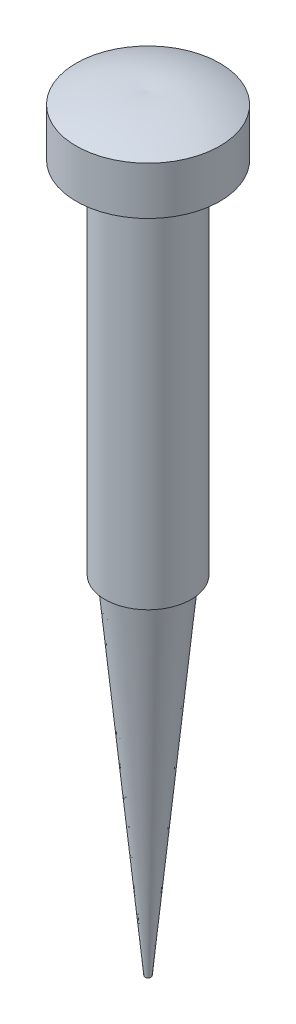
SolidWorks part; units mm, degrees
material "Plain Carbon Steel"
ref_plane "Front Plane" through (0, 0, 0) normal (0, 0, 1) x (1, 0, 0)
ref_plane "Top Plane" through (0, 0, 0) normal (0, 1, 0) x (1, 0, 0)
ref_plane "Right Plane" through (0, 0, 0) normal (1, 0, 0) x (0, 0, -1)
sketch "Head and Stem Profile" plane through (0, 0, 0) normal (0, 0, 1) x (1, 0, 0)
  line L0 (0, 0) -> (0, 17.5)
  line L2 (3, 17) -> (3, 15)
  line L3 (3, 15) -> (1.8, 15)
  line L4 (1.8, 15) -> (1.8, 0)
  line L6 (1.8, 0) -> (0, 0)
  arc A0 (3, 17) -> (0, 17.5) centre (0.5458, 11.5249) ccw
  dimension "D4" = 6
  dimension "D1" = 15
  dimension "D2" = 2
  dimension "D3" = 0.5
  dimension "D5" = 3
  dimension "D6" = 1.8
  dimension "D9" = 1.8
revolve "Head and Stem Revolve" add sketch "Head and Stem Profile" angle 360 about L0
sketch "Tip Base Circle Ø3" plane through (0, 0, 0) normal (0, -1, 0) x (1, 0, 0)
  circle A0 centre (0, 0) radius 1.5
  dimension "D1" = 3
extrude "Tapered Needle Tip" add sketch "Tip Base Circle Ø3" along normal blind 14.5 draft 5.42
